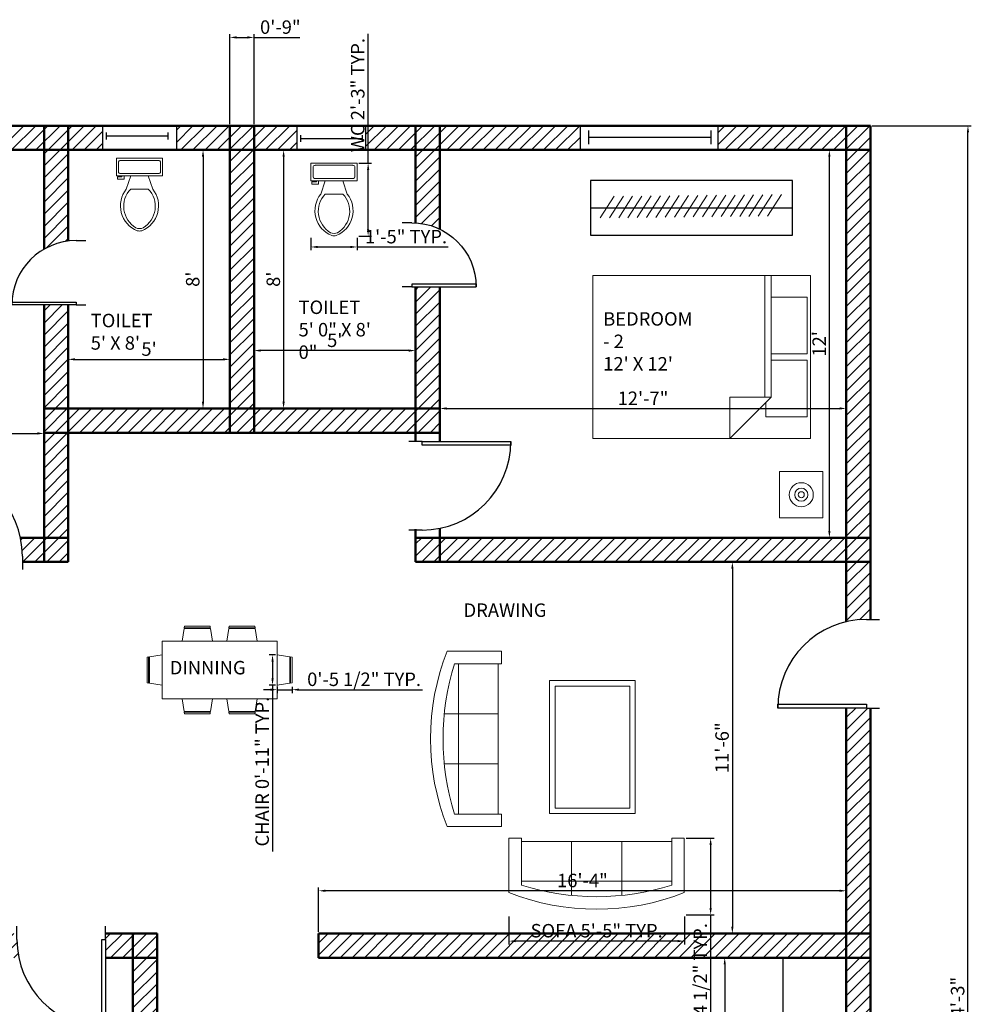
# Model space of a CAD drawing. Units: millimetres. Extents: x 2829 to 4029, y 962 to 1687.
# Tile 7 of 7: x 3676 to 4029, y 1321 to 1687. Entities that reach past the tile are written whole.
import ezdxf

# ---------------------------------------------------------------- set-up
doc = ezdxf.new("R2010")
doc.units = ezdxf.units.MM
for name, color, linetype, lineweight in [('A-ANNO-DIMS', 140, 'Continuous', 18), ('A-AREA-IDEN', 190, 'Continuous', 25), ('A-FLOR-CASE', 90, 'Continuous', 25), ('A-FLOR-CASE-PATT', 90, 'Continuous', 13), ('A-FLOR-FIXT', 90, 'Continuous', 18), ('A-WALL-PATT', 2, 'Continuous', 13), ('doors', 10, 'Continuous', 25), ('furniture', 90, 'Continuous', 18), ('walls', 50, 'Continuous', 50), ('windows', 30, 'Continuous', 25)]:
    doc.layers.add(name, color=color, linetype=linetype, lineweight=lineweight)
doc.styles.get("Standard").update_dxf_attribs({"font": 'arial.ttf'})
doc.dimstyles.new('ISO-25', dxfattribs={"dimtxt": 5, "dimasz": 2.5, "dimexe": 1.25, "dimexo": 0.625, "dimtad": 1, "dimdec": 0, "dimlunit": 3, "dimtxsty": 'Standard', "dimcen": 2.5, "dimadec": 0, "dimazin": 0, "dimtfac": 1, "dimtdec": 0, "dimtmove": 0, "dimatfit": 3, "dimfxl": 1, "dimarcsym": 0})
pattern_1 = [(45, (-1090.0668, 570.9627), (-2.245064, 2.245064), [])]

# ---------------------------------------------------------------- blocks, each defined once
blk = doc.blocks.new('*U2')
for p, q in [((0, 0), (0, -6)), ((40, 0), (40, -6))]:
    blk.add_line(p, q)
blk.add_lwpolyline([(0, 0), (0, 40), (1.75, 40), (1.75, 0)], close=True)
blk.add_arc((0, 0), 40, 0, 90)
blk = doc.blocks.new('*U32')
for p, q in [((0, 4), (0, 0)), ((36, 4), (36, 0)), ((0, 2), (36, 2))]:
    blk.add_line(p, q)
blk = doc.blocks.new('*U33')
for p, q in [((0, 4), (0, 0)), ((0, 2), (36, 2)), ((36, 4), (36, 0))]:
    blk.add_line(p, q)
blk = doc.blocks.new('Bed - Queen')
for p, q in [((0, -80.00003), (0, 0)), ((0, 0), (59.99999, 0)), ((59.99999, 0), (59.99999, -80.00003)), ((7.99999, -1.2), (28.79998, -1.2)), ((7.99999, -14.4), (7.99999, -1.2)), ((28.79998, -1.2), (28.79998, -14.4)), ((31.19999, -1.2), (51.99999, -1.2)), ((31.19999, -14.4), (31.19999, -1.2)), ((51.99999, -1.2), (51.99999, -16.4)), ((0, -14.4), (44.8, -14.4)), ((59.99999, -29.6), (44.8, -14.4)), ((44.8, -14.4), (44.8, -29.6)), ((44.8, -16.8), (0, -16.8)), ((51.99999, -16.4), (46.79936, -16.4)), ((44.8, -29.6), (59.99999, -29.6)), ((59.99999, -80.00003), (0, -80.00003))]:
    blk.add_line(p, q)
blk = doc.blocks.new('Sofa - Roundback 7 ft.')
for p, q in [((-12.00002, -32.4421), (-12.00003, -6.5971)), ((11.99997, -32.4421), (11.99998, -6.5971)), ((-36.000027, -34), (-36.000027, -11.4696)), ((-35.999844, -13.3819), (35.9998, -13.3819)), ((35.99998, -34), (35.99998, -11.4696)), ((-36.000027, -32.4421), (35.99998, -32.4421))]:
    blk.add_line(p, q)
for points in [[(-36.000027, -34), (-42.000027, -34), (-42.000027, -8)], [(41.99998, -8), (41.99998, -34), (35.99998, -34)]]:
    blk.add_lwpolyline(points)
for centre, radius, start, end in [((0, -114.25), 114.25, 68.43141, 111.5686), ((-0.00001, -127.1968), 121.1968, 72.72033, 107.2797)]:
    blk.add_arc(centre, radius, start, end)
blk = doc.blocks.new('Toilet - top')
for p, q in [((9.5, -6), (9.5, -2)), ((-10, -8.5), (-8, -8.5)), ((-10, -9.5), (-10, -8.5)), ((-8, -8.5), (-8, -8)), ((-7, -8), (-7, -9.5)), ((-4, -8), (-6, -14)), ((4, -8), (6, -14)), ((-7, -9.5), (-10, -9.5)), ((4, -14), (-4, -14))]:
    blk.add_line(p, q)
blk.add_lwpolyline([(10.5, -8), (10.5, 0), (-10.5, 0), (-10.5, -8)], close=True)
for points in [[(-9.5, -2), (-9.5, -6)], [(8.5, -1), (-8.5, -1)], [(-8.5, -7), (8.5, -7)]]:
    blk.add_lwpolyline(points)
for centre, radius, start, end in [((-8.62, -1.88), 0.884, 81.8699, 188.1301), ((8.62, -1.88), 0.884, 351.8699, 98.1301), ((-8.62, -6.12), 0.884, 171.8699, 278.1301), ((8.62, -6.12), 0.884, 261.8699, 8.1301), ((3.52, -21.58), 12.17, 141.4691, 247.9714), ((4.2, -21.82), 11.33, 136.3677, 238.9468), ((-3.52, -21.58), 12.17, 292.0284, 38.5307), ((-4.2, -21.82), 11.33, 301.053, 43.6321), ((0, -27.88), 4, 245.7318, 294.2682), ((0, -29), 4, 254.8605, 285.1395)]:
    blk.add_arc(centre, radius, start, end)
blk = doc.blocks.new('*D36')
at = {"layer": 'A-ANNO-DIMS', "color": 0, "lineweight": -2, "transparency": 16777216}
for p, q in [((3533.66, 1539.68), (3533.66, 1531.75)), ((3684.66, 1539.68), (3684.66, 1531.75)), ((3536.16, 1533), (3682.16, 1533))]:
    blk.add_line(p, q, dxfattribs=at)
at = {"layer": 'A-ANNO-DIMS', "color": 0, "transparency": 16777216}
for points in [[(3536.16, 1533.42), (3536.16, 1532.59), (3533.66, 1533)], [(3682.16, 1533.42), (3682.16, 1532.59), (3684.66, 1533)]]:
    blk.add_solid(points, dxfattribs=at)
at = {"layer": 'Defpoints', "color": 0, "transparency": 16777216}
for p in [(3533.66, 1540.3), (3684.66, 1540.3), (3684.66, 1533)]:
    blk.add_point(p, dxfattribs=at)
at = {"layer": 'A-ANNO-DIMS', "color": 0, "transparency": 16777216, "insert": (3609.16, 1536.14), "char_height": 5, "attachment_point": 5}
blk.add_mtext('12\'-7"', dxfattribs=at)
blk = doc.blocks.new('*D38')
at = {"layer": 'A-ANNO-DIMS', "color": 0, "lineweight": -2, "transparency": 16777216}
for p, q in [((3744.35, 1638.27), (3744.97, 1638.27)), ((3743.72, 1635.77), (3743.72, 1544.77)), ((3744.35, 1542.27), (3744.97, 1542.27))]:
    blk.add_line(p, q, dxfattribs=at)
at = {"layer": 'A-ANNO-DIMS', "color": 0, "transparency": 16777216}
for points in [[(3743.3, 1635.77), (3744.14, 1635.77), (3743.72, 1638.27)], [(3743.3, 1544.77), (3744.14, 1544.77), (3743.72, 1542.27)]]:
    blk.add_solid(points, dxfattribs=at)
at = {"layer": 'Defpoints', "color": 0, "transparency": 16777216}
for p in [(3743.72, 1638.27), (3743.72, 1542.27), (3743.72, 1542.27)]:
    blk.add_point(p, dxfattribs=at)
at = {"layer": 'A-ANNO-DIMS', "color": 0, "transparency": 16777216, "insert": (3740.54, 1590.27), "char_height": 5, "attachment_point": 5, "rotation": 90}
blk.add_mtext("8'", dxfattribs=at)
blk = doc.blocks.new('*D39')
at = {"layer": 'A-ANNO-DIMS', "color": 0, "lineweight": -2, "transparency": 16777216}
for p, q in [((3693.66, 1556.42), (3693.66, 1561.76)), ((3753.66, 1556.42), (3753.66, 1561.76)), ((3696.16, 1560.51), (3751.16, 1560.51))]:
    blk.add_line(p, q, dxfattribs=at)
at = {"layer": 'A-ANNO-DIMS', "color": 0, "transparency": 16777216}
for points in [[(3696.16, 1560.92), (3696.16, 1560.09), (3693.66, 1560.51)], [(3751.16, 1560.92), (3751.16, 1560.09), (3753.66, 1560.51)]]:
    blk.add_solid(points, dxfattribs=at)
at = {"layer": 'Defpoints', "color": 0, "transparency": 16777216}
for p in [(3753.66, 1560.51), (3693.66, 1555.8), (3753.66, 1555.8)]:
    blk.add_point(p, dxfattribs=at)
at = {"layer": 'A-ANNO-DIMS', "color": 0, "transparency": 16777216, "insert": (3723.66, 1563.67), "char_height": 5, "attachment_point": 5}
blk.add_mtext("5'", dxfattribs=at)
blk = doc.blocks.new('*D40')
at = {"layer": 'A-ANNO-DIMS', "color": 0, "lineweight": -2, "transparency": 16777216}
for p, q in [((3774.27, 1638.27), (3774.9, 1638.27)), ((3773.65, 1635.77), (3773.65, 1544.77)), ((3774.27, 1542.27), (3774.9, 1542.27))]:
    blk.add_line(p, q, dxfattribs=at)
at = {"layer": 'A-ANNO-DIMS', "color": 0, "transparency": 16777216}
for points in [[(3773.23, 1635.77), (3774.07, 1635.77), (3773.65, 1638.27)], [(3773.23, 1544.77), (3774.07, 1544.77), (3773.65, 1542.27)]]:
    blk.add_solid(points, dxfattribs=at)
at = {"layer": 'Defpoints', "color": 0, "transparency": 16777216}
for p in [(3773.65, 1638.27), (3773.65, 1542.27), (3773.65, 1542.27)]:
    blk.add_point(p, dxfattribs=at)
at = {"layer": 'A-ANNO-DIMS', "color": 0, "transparency": 16777216, "insert": (3770.47, 1590.27), "char_height": 5, "attachment_point": 5, "rotation": 90}
blk.add_mtext("8'", dxfattribs=at)
blk = doc.blocks.new('*D41')
at = {"layer": 'A-ANNO-DIMS', "color": 0, "lineweight": -2, "transparency": 16777216}
for p, q in [((3762.66, 1564.4), (3762.66, 1565.02)), ((3820.16, 1563.77), (3765.16, 1563.77)), ((3822.66, 1564.4), (3822.66, 1565.02))]:
    blk.add_line(p, q, dxfattribs=at)
at = {"layer": 'A-ANNO-DIMS', "color": 0, "transparency": 16777216}
for points in [[(3765.16, 1564.19), (3765.16, 1563.35), (3762.66, 1563.77)], [(3820.16, 1564.19), (3820.16, 1563.35), (3822.66, 1563.77)]]:
    blk.add_solid(points, dxfattribs=at)
at = {"layer": 'Defpoints', "color": 0, "transparency": 16777216}
for p in [(3762.66, 1563.77), (3762.66, 1563.77), (3822.66, 1563.77)]:
    blk.add_point(p, dxfattribs=at)
at = {"layer": 'A-ANNO-DIMS', "color": 0, "transparency": 16777216, "insert": (3792.66, 1566.94), "char_height": 5, "attachment_point": 5}
blk.add_mtext("5'", dxfattribs=at)
blk = doc.blocks.new('*D53')
at = {"layer": 'A-ANNO-DIMS', "color": 0, "lineweight": -2, "transparency": 16777216}
for p, q in [((3940.98, 1485.27), (3941.6, 1485.27)), ((3940.35, 1482.77), (3940.35, 1349.77)), ((3940.98, 1347.27), (3941.6, 1347.27))]:
    blk.add_line(p, q, dxfattribs=at)
at = {"layer": 'A-ANNO-DIMS', "color": 0, "transparency": 16777216}
for points in [[(3939.94, 1482.77), (3940.77, 1482.77), (3940.35, 1485.27)], [(3939.94, 1349.77), (3940.77, 1349.77), (3940.35, 1347.27)]]:
    blk.add_solid(points, dxfattribs=at)
at = {"layer": 'Defpoints', "color": 0, "transparency": 16777216}
for p in [(3940.35, 1485.27), (3940.35, 1347.27), (3940.35, 1347.27)]:
    blk.add_point(p, dxfattribs=at)
at = {"layer": 'A-ANNO-DIMS', "color": 0, "transparency": 16777216, "insert": (3937.17, 1416.27), "char_height": 5, "attachment_point": 5, "rotation": 90}
blk.add_mtext('11\'-6"', dxfattribs=at)
blk = doc.blocks.new('*D54')
at = {"layer": 'A-ANNO-DIMS', "color": 0, "lineweight": -2, "transparency": 16777216}
for p, q in [((3786.66, 1347.9), (3786.66, 1364.4)), ((3982.66, 1354.73), (3982.66, 1364.4)), ((3980.16, 1363.15), (3789.16, 1363.15))]:
    blk.add_line(p, q, dxfattribs=at)
at = {"layer": 'A-ANNO-DIMS', "color": 0, "transparency": 16777216}
for points in [[(3789.16, 1363.56), (3789.16, 1362.73), (3786.66, 1363.15)], [(3980.16, 1363.56), (3980.16, 1362.73), (3982.66, 1363.15)]]:
    blk.add_solid(points, dxfattribs=at)
at = {"layer": 'Defpoints', "color": 0, "transparency": 16777216}
for p in [(3786.66, 1363.15), (3982.66, 1354.11), (3786.66, 1347.27)]:
    blk.add_point(p, dxfattribs=at)
at = {"layer": 'A-ANNO-DIMS', "color": 0, "transparency": 16777216, "insert": (3884.66, 1366.32), "char_height": 5, "attachment_point": 5}
blk.add_mtext('16\'-4"', dxfattribs=at)
blk = doc.blocks.new('*D55')
at = {"layer": 'A-ANNO-DIMS', "color": 0, "lineweight": -2, "transparency": 16777216}
for p, q in [((3937.54, 1338.27), (3936.26, 1338.27)), ((3937.51, 1335.77), (3937.51, 1196.77)), ((3937.54, 1194.27), (3936.26, 1194.27))]:
    blk.add_line(p, q, dxfattribs=at)
at = {"layer": 'A-ANNO-DIMS', "color": 0, "transparency": 16777216}
for points in [[(3937.1, 1335.77), (3937.93, 1335.77), (3937.51, 1338.27)], [(3937.1, 1196.77), (3937.93, 1196.77), (3937.51, 1194.27)]]:
    blk.add_solid(points, dxfattribs=at)
at = {"layer": 'Defpoints', "color": 0, "transparency": 16777216}
for p in [(3938.16, 1338.27), (3937.51, 1194.27), (3938.16, 1194.27)]:
    blk.add_point(p, dxfattribs=at)
at = {"layer": 'A-ANNO-DIMS', "color": 0, "transparency": 16777216, "insert": (3934.38, 1266.27), "char_height": 5, "attachment_point": 5, "rotation": 90}
blk.add_mtext("12'", dxfattribs=at)
blk = doc.blocks.new('*D57')
at = {"layer": 'A-ANNO-DIMS', "color": 0, "lineweight": -2, "transparency": 16777216}
for p, q in [((3977.01, 1638.27), (3977.64, 1638.27)), ((3976.39, 1496.77), (3976.39, 1635.77)), ((3977.01, 1494.27), (3977.64, 1494.27))]:
    blk.add_line(p, q, dxfattribs=at)
at = {"layer": 'A-ANNO-DIMS', "color": 0, "transparency": 16777216}
for points in [[(3975.97, 1635.77), (3976.81, 1635.77), (3976.39, 1638.27)], [(3975.97, 1496.77), (3976.81, 1496.77), (3976.39, 1494.27)]]:
    blk.add_solid(points, dxfattribs=at)
at = {"layer": 'Defpoints', "color": 0, "transparency": 16777216}
for p in [(3976.39, 1638.27), (3976.39, 1638.27), (3976.39, 1494.27)]:
    blk.add_point(p, dxfattribs=at)
at = {"layer": 'A-ANNO-DIMS', "color": 0, "transparency": 16777216, "insert": (3973.25, 1566.27), "char_height": 5, "attachment_point": 5, "rotation": 90}
blk.add_mtext("12'", dxfattribs=at)
blk = doc.blocks.new('*D58')
at = {"layer": 'A-ANNO-DIMS', "color": 0, "lineweight": -2, "transparency": 16777216}
for p, q in [((3831.66, 1542.9), (3831.66, 1543.52)), ((3982.66, 1542.9), (3982.66, 1543.52)), ((3834.16, 1542.27), (3980.16, 1542.27))]:
    blk.add_line(p, q, dxfattribs=at)
at = {"layer": 'A-ANNO-DIMS', "color": 0, "transparency": 16777216}
for points in [[(3834.16, 1542.69), (3834.16, 1541.85), (3831.66, 1542.27)], [(3980.16, 1542.69), (3980.16, 1541.85), (3982.66, 1542.27)]]:
    blk.add_solid(points, dxfattribs=at)
at = {"layer": 'Defpoints', "color": 0, "transparency": 16777216}
for p in [(3831.66, 1542.27), (3982.66, 1542.27), (3982.66, 1542.27)]:
    blk.add_point(p, dxfattribs=at)
at = {"layer": 'A-ANNO-DIMS', "color": 0, "transparency": 16777216, "insert": (3907.16, 1545.41), "char_height": 5, "attachment_point": 5}
blk.add_mtext('12\'-7"', dxfattribs=at)
blk = doc.blocks.new('CHAIR-DINING')
for p, q in [((0.74, 4.74), (0, 0)), ((0.74, 4.74), (10.5, 4.74)), ((0.88, 5.63), (0.79, 5.04)), ((10.46, 5.04), (0.79, 5.04)), ((0.88, 5.63), (10.36, 5.63)), ((10.46, 5.04), (10.36, 5.63)), ((11.24, 0), (10.5, 4.74))]:
    blk.add_line(p, q)
blk = doc.blocks.new('*D67')
at = {"layer": 'A-ANNO-DIMS', "color": 0, "lineweight": -2, "transparency": 16777216}
for p, q in [((3857.36, 1353.61), (3857.36, 1343.21)), ((3922.51, 1353.61), (3922.51, 1343.21)), ((3920.01, 1344.46), (3859.86, 1344.46))]:
    blk.add_line(p, q, dxfattribs=at)
at = {"layer": 'A-ANNO-DIMS', "color": 0, "transparency": 16777216}
for points in [[(3859.86, 1344.88), (3859.86, 1344.04), (3857.36, 1344.46)], [(3920.01, 1344.88), (3920.01, 1344.04), (3922.51, 1344.46)]]:
    blk.add_solid(points, dxfattribs=at)
at = {"layer": 'Defpoints', "color": 0, "transparency": 16777216}
for p in [(3857.36, 1354.23), (3922.51, 1354.23), (3857.36, 1344.46)]:
    blk.add_point(p, dxfattribs=at)
at = {"layer": 'A-ANNO-DIMS', "color": 0, "transparency": 16777216, "insert": (3889.93, 1347.67), "char_height": 5, "attachment_point": 5}
blk.add_mtext('SOFA 5\'-5" TYP.', dxfattribs=at)
blk = doc.blocks.new('*D68')
at = {"layer": 'A-ANNO-DIMS', "color": 0, "lineweight": -2, "transparency": 16777216}
for p, q in [((3923.13, 1382.67), (3933.53, 1382.67)), ((3932.28, 1380.17), (3932.28, 1356.73)), ((3923.13, 1354.23), (3933.53, 1354.23)), ((3932.28, 1354.23), (3932.28, 1308.27))]:
    blk.add_line(p, q, dxfattribs=at)
at = {"layer": 'A-ANNO-DIMS', "color": 0, "transparency": 16777216}
for points in [[(3931.86, 1380.17), (3932.7, 1380.17), (3932.28, 1382.67)], [(3931.86, 1356.73), (3932.7, 1356.73), (3932.28, 1354.23)]]:
    blk.add_solid(points, dxfattribs=at)
at = {"layer": 'Defpoints', "color": 0, "transparency": 16777216}
for p in [(3922.51, 1382.67), (3922.51, 1354.23), (3932.28, 1354.23)]:
    blk.add_point(p, dxfattribs=at)
at = {"layer": 'A-ANNO-DIMS', "color": 0, "transparency": 16777216, "insert": (3929.07, 1330), "char_height": 5, "attachment_point": 5, "rotation": 90}
blk.add_mtext('2\'-4 1/2" TYP.', dxfattribs=at)
blk = doc.blocks.new('*D75')
at = {"layer": 'A-ANNO-DIMS', "color": 0, "lineweight": -2, "transparency": 16777216}
for p, q in [((3805.04, 1633.39), (3805.04, 1681.4)), ((3801.61, 1633.39), (3806.29, 1633.39)), ((3805.04, 1608.81), (3805.04, 1630.89)), ((3801.61, 1606.31), (3806.29, 1606.31))]:
    blk.add_line(p, q, dxfattribs=at)
at = {"layer": 'A-ANNO-DIMS', "color": 0, "transparency": 16777216}
for points in [[(3804.63, 1630.89), (3805.46, 1630.89), (3805.04, 1633.39)], [(3804.63, 1608.81), (3805.46, 1608.81), (3805.04, 1606.31)]]:
    blk.add_solid(points, dxfattribs=at)
at = {"layer": 'Defpoints', "color": 0, "transparency": 16777216}
for p in [(3800.98, 1633.39), (3805.04, 1633.39), (3800.98, 1606.31)]:
    blk.add_point(p, dxfattribs=at)
at = {"layer": 'A-ANNO-DIMS', "color": 0, "transparency": 16777216, "insert": (3801.83, 1658.65), "char_height": 5, "attachment_point": 5, "rotation": 90}
blk.add_mtext('WC 2\'-3" TYP.', dxfattribs=at)
blk = doc.blocks.new('*D76')
at = {"layer": 'A-ANNO-DIMS', "color": 0, "lineweight": -2, "transparency": 16777216}
for p, q in [((3783.78, 1605.69), (3783.78, 1601)), ((3800.98, 1605.69), (3800.98, 1601)), ((3786.28, 1602.25), (3798.48, 1602.25)), ((3800.98, 1602.25), (3834.74, 1602.25))]:
    blk.add_line(p, q, dxfattribs=at)
at = {"layer": 'A-ANNO-DIMS', "color": 0, "transparency": 16777216}
for points in [[(3786.28, 1602.67), (3786.28, 1601.84), (3783.78, 1602.25)], [(3798.48, 1602.67), (3798.48, 1601.84), (3800.98, 1602.25)]]:
    blk.add_solid(points, dxfattribs=at)
at = {"layer": 'Defpoints', "color": 0, "transparency": 16777216}
for p in [(3783.78, 1606.31), (3800.98, 1606.31), (3800.98, 1602.25)]:
    blk.add_point(p, dxfattribs=at)
at = {"layer": 'A-ANNO-DIMS', "color": 0, "transparency": 16777216, "insert": (3819.11, 1605.43), "char_height": 5, "attachment_point": 5}
blk.add_mtext('1\'-5" TYP.', dxfattribs=at)
blk = doc.blocks.new('*D77')
at = {"layer": 'A-ANNO-DIMS', "color": 0, "lineweight": -2, "transparency": 16777216}
for p, q in [((3770.6, 1450.76), (3768.29, 1450.76)), ((3769.54, 1448.26), (3769.54, 1442.01)), ((3770.6, 1439.51), (3768.29, 1439.51)), ((3769.54, 1439.51), (3769.54, 1377.78))]:
    blk.add_line(p, q, dxfattribs=at)
at = {"layer": 'A-ANNO-DIMS', "color": 0, "transparency": 16777216}
for points in [[(3769.13, 1448.26), (3769.96, 1448.26), (3769.54, 1450.76)], [(3769.13, 1442.01), (3769.96, 1442.01), (3769.54, 1439.51)]]:
    blk.add_solid(points, dxfattribs=at)
at = {"layer": 'Defpoints', "color": 0, "transparency": 16777216}
for p in [(3771.23, 1450.76), (3769.54, 1439.51), (3771.23, 1439.51)]:
    blk.add_point(p, dxfattribs=at)
at = {"layer": 'A-ANNO-DIMS', "color": 0, "transparency": 16777216, "insert": (3766.33, 1407.4), "char_height": 5, "attachment_point": 5, "rotation": 90}
blk.add_mtext('CHAIR 0\'-11" TYP.', dxfattribs=at)
blk = doc.blocks.new('*D78')
at = {"layer": 'A-ANNO-DIMS', "color": 0, "lineweight": -2, "transparency": 16777216}
for p, q in [((3768.73, 1437.83), (3766.23, 1437.83)), ((3771.23, 1438.89), (3771.23, 1436.58)), ((3771.23, 1437.83), (3776.86, 1437.83)), ((3776.86, 1438.89), (3776.86, 1436.58)), ((3779.36, 1437.83), (3825.24, 1437.83))]:
    blk.add_line(p, q, dxfattribs=at)
at = {"layer": 'A-ANNO-DIMS', "color": 0, "transparency": 16777216}
for points in [[(3768.73, 1438.24), (3768.73, 1437.41), (3771.23, 1437.83)], [(3779.36, 1438.24), (3779.36, 1437.41), (3776.86, 1437.83)]]:
    blk.add_solid(points, dxfattribs=at)
at = {"layer": 'Defpoints', "color": 0, "transparency": 16777216}
for p in [(3771.23, 1439.51), (3776.86, 1439.51), (3776.86, 1437.83)]:
    blk.add_point(p, dxfattribs=at)
at = {"layer": 'A-ANNO-DIMS', "color": 0, "transparency": 16777216, "insert": (3803.55, 1441.04), "char_height": 5, "attachment_point": 5}
blk.add_mtext('0\'-5 1/2" TYP.', dxfattribs=at)
blk = doc.blocks.new('*D92')
at = {"layer": 'A-ANNO-DIMS', "color": 0, "lineweight": -2, "transparency": 16777216}
for p, q in [((3443.66, 1337.65), (3443.66, 962.22)), ((3991.66, 995.65), (3991.66, 962.22)), ((3446.16, 963.47), (3989.16, 963.47))]:
    blk.add_line(p, q, dxfattribs=at)
at = {"layer": 'A-ANNO-DIMS', "color": 0, "transparency": 16777216}
for points in [[(3446.16, 963.89), (3446.16, 963.05), (3443.66, 963.47)], [(3989.16, 963.89), (3989.16, 963.05), (3991.66, 963.47)]]:
    blk.add_solid(points, dxfattribs=at)
at = {"layer": 'Defpoints', "color": 0, "transparency": 16777216}
for p in [(3443.66, 1338.27), (3991.66, 996.27), (3991.66, 963.47)]:
    blk.add_point(p, dxfattribs=at)
at = {"layer": 'A-ANNO-DIMS', "color": 0, "transparency": 16777216, "insert": (3717.66, 966.65), "char_height": 5, "attachment_point": 5}
blk.add_mtext('45\'-8"', dxfattribs=at)
blk = doc.blocks.new('*D93')
at = {"layer": 'A-ANNO-DIMS', "color": 0, "lineweight": -2, "transparency": 16777216}
for p, q in [((3992.28, 1647.27), (4029.11, 1647.27)), ((4027.86, 998.77), (4027.86, 1644.77)), ((3992.28, 996.27), (4029.11, 996.27))]:
    blk.add_line(p, q, dxfattribs=at)
at = {"layer": 'A-ANNO-DIMS', "color": 0, "transparency": 16777216}
for points in [[(4027.44, 1644.77), (4028.28, 1644.77), (4027.86, 1647.27)], [(4027.44, 998.77), (4028.28, 998.77), (4027.86, 996.27)]]:
    blk.add_solid(points, dxfattribs=at)
at = {"layer": 'Defpoints', "color": 0, "transparency": 16777216}
for p in [(3991.66, 1647.27), (4027.86, 1647.27), (3991.66, 996.27)]:
    blk.add_point(p, dxfattribs=at)
at = {"layer": 'A-ANNO-DIMS', "color": 0, "transparency": 16777216, "insert": (4024.68, 1321.77), "char_height": 5, "attachment_point": 5, "rotation": 90}
blk.add_mtext('54\'-3"', dxfattribs=at)
blk = doc.blocks.new('*D95')
at = {"layer": 'A-ANNO-DIMS', "color": 0, "lineweight": -2, "transparency": 16777216}
for p, q in [((3753.66, 1647.9), (3753.66, 1681.32)), ((3756.16, 1680.07), (3760.16, 1680.07)), ((3762.66, 1647.9), (3762.66, 1681.32)), ((3762.66, 1680.07), (3779.7, 1680.07))]:
    blk.add_line(p, q, dxfattribs=at)
at = {"layer": 'A-ANNO-DIMS', "color": 0, "transparency": 16777216}
for points in [[(3756.16, 1680.49), (3756.16, 1679.65), (3753.66, 1680.07)], [(3760.16, 1680.49), (3760.16, 1679.65), (3762.66, 1680.07)]]:
    blk.add_solid(points, dxfattribs=at)
at = {"layer": 'Defpoints', "color": 0, "transparency": 16777216}
for p in [(3762.66, 1680.07), (3753.66, 1647.27), (3762.66, 1647.27)]:
    blk.add_point(p, dxfattribs=at)
at = {"layer": 'A-ANNO-DIMS', "color": 0, "transparency": 16777216, "insert": (3772.43, 1683.25), "char_height": 5, "attachment_point": 5}
blk.add_mtext('0\'-9"', dxfattribs=at)

msp = doc.modelspace()

# ---------------------------------------------------------------- hatches: boundary and pattern name
at = {"layer": 'A-FLOR-CASE-PATT'}
h = msp.add_hatch(dxfattribs=at)
h.set_pattern_fill('ANSI31', color=256, scale=0.908318, angle=12.144, style=0)
h.paths.add_polyline_path([(3889.26, 1612.99), (3954.95, 1613.71), (3960.15, 1621.75), (3894.46, 1621.04)])
at = {"layer": 'A-WALL-PATT'}
h = msp.add_hatch(dxfattribs=at)
h.set_pattern_fill('ANSI31', color=256)
h.set_pattern_definition(pattern_1)
h.paths.add_polyline_path([(3524.66, 1494.27), (3452.66, 1494.27), (3452.66, 1485.27), (3524.66, 1485.27)])
h.paths.add_polyline_path([(3452.66, 1494.27), (3443.66, 1494.27), (3443.66, 1485.27), (3452.66, 1485.27)])
h.paths.add_polyline_path([(3452.66, 1485.27), (3443.66, 1485.27), (3443.66, 1347.27), (3452.66, 1347.27)])
h.paths.add_polyline_path([(3533.66, 1433.28), (3524.66, 1433.28), (3524.66, 1400.41), (3533.66, 1400.41)])
h.paths.add_polyline_path([(3524.66, 1347.27), (3452.66, 1347.27), (3452.66, 1338.27), (3524.66, 1338.27)])
h.paths.add_polyline_path([(3452.66, 1347.27), (3443.66, 1347.27), (3443.66, 1338.27), (3452.66, 1338.27)])
h.paths.add_polyline_path([(3533.66, 1347.27), (3524.66, 1347.27), (3524.66, 1338.27), (3533.66, 1338.27)])
h.paths.add_polyline_path([(3674.61, 1345.02), (3674.61, 1347.27), (3533.66, 1347.27), (3533.66, 1338.27), (3675.31, 1338.27, -0.051672)])
h.paths.add_polyline_path([(3533.66, 1638.27), (3524.66, 1638.27), (3524.66, 1494.27), (3533.66, 1494.27)])
h.paths.add_polyline_path([(3533.66, 1494.27), (3524.66, 1494.27), (3524.66, 1485.27), (3533.66, 1485.27)])
h.paths.add_polyline_path([(3643.72, 1494.27), (3533.66, 1494.27), (3533.66, 1485.27), (3643.72, 1485.27), (3643.72, 1487.41)])
h.paths.add_polyline_path([(3533.66, 1647.27), (3524.66, 1647.27), (3524.66, 1638.27), (3533.66, 1638.27)])
h.paths.add_polyline_path([(3573.07, 1647.27), (3533.66, 1647.27), (3533.66, 1638.27), (3573.07, 1638.27)])
h.paths.add_polyline_path([(3684.66, 1647.27), (3622.32, 1647.27), (3622.32, 1638.27), (3684.66, 1638.27)])
h.paths.add_polyline_path([(3693.66, 1647.27), (3684.66, 1647.27), (3684.66, 1638.27), (3693.66, 1638.27)])
h.paths.add_polyline_path([(3693.66, 1638.27), (3684.66, 1638.27), (3684.66, 1601.42, -0.100401), (3693.66, 1604.42)])
h.paths.add_polyline_path([(3693.66, 1580.73), (3684.66, 1580.73), (3684.66, 1542.27), (3693.66, 1542.27)])
h.paths.add_polyline_path([(3693.66, 1542.27), (3684.66, 1542.27), (3684.66, 1533.27), (3693.66, 1533.27)])
h.paths.add_polyline_path([(3693.66, 1533.27), (3684.66, 1533.27), (3684.66, 1494.27), (3693.66, 1494.27)])
h.paths.add_polyline_path([(3693.66, 1494.27), (3684.66, 1494.27), (3684.66, 1485.27), (3693.66, 1485.27)])
h.paths.add_polyline_path([(3684.66, 1494.27), (3675.91, 1494.27, -0.052559), (3676.64, 1487.41), (3676.64, 1485.27), (3684.66, 1485.27)])
h.paths.add_polyline_path([(3753.66, 1542.27), (3693.66, 1542.27), (3693.66, 1533.27), (3753.66, 1533.27)])
h.paths.add_polyline_path([(3762.66, 1542.27), (3753.66, 1542.27), (3753.66, 1533.27), (3762.66, 1533.27)])
h.paths.add_polyline_path([(3762.66, 1638.27), (3753.66, 1638.27), (3753.66, 1542.27), (3762.66, 1542.27)])
h.paths.add_polyline_path([(3762.66, 1647.27), (3753.66, 1647.27), (3753.66, 1638.27), (3762.66, 1638.27)])
h.paths.add_polyline_path([(3753.66, 1647.27), (3733.82, 1647.27), (3733.82, 1638.27), (3753.66, 1638.27)])
h.paths.add_polyline_path([(3706.41, 1647.27), (3693.66, 1647.27), (3693.66, 1638.27), (3706.41, 1638.27)])
h.paths.add_polyline_path([(3822.66, 1647.27), (3804.07, 1647.27), (3804.07, 1638.27), (3822.66, 1638.27)])
h.paths.add_polyline_path([(3778.61, 1647.27), (3762.66, 1647.27), (3762.66, 1638.27), (3778.61, 1638.27)])
h.paths.add_polyline_path([(3822.66, 1542.27), (3762.66, 1542.27), (3762.66, 1533.27), (3822.66, 1533.27)])
h.paths.add_polyline_path([(3831.66, 1542.27), (3822.66, 1542.27), (3822.66, 1533.27), (3831.66, 1533.27)])
h.paths.add_polyline_path([(3831.66, 1587.4), (3822.66, 1587.4), (3822.66, 1542.27), (3831.66, 1542.27)])
h.paths.add_polyline_path([(3831.66, 1638.27), (3822.66, 1638.27), (3822.66, 1611.22, -0.098322), (3831.66, 1608.9)])
h.paths.add_polyline_path([(3831.66, 1647.27), (3822.66, 1647.27), (3822.66, 1638.27), (3831.66, 1638.27)])
h.paths.add_polyline_path([(3883.77, 1647.27), (3831.66, 1647.27), (3831.66, 1638.27), (3883.77, 1638.27)])
h.paths.add_polyline_path([(3982.66, 1647.27), (3934.96, 1647.27), (3934.96, 1638.27), (3982.66, 1638.27)])
h.paths.add_polyline_path([(3991.66, 1647.27), (3982.66, 1647.27), (3982.66, 1638.27), (3991.66, 1638.27)])
h.paths.add_polyline_path([(3991.66, 1638.27), (3982.66, 1638.27), (3982.66, 1494.27), (3991.66, 1494.27)])
h.paths.add_polyline_path([(3991.66, 1494.27), (3982.66, 1494.27), (3982.66, 1485.27), (3991.66, 1485.27)])
h.paths.add_polyline_path([(3982.66, 1494.27), (3831.66, 1494.27), (3831.66, 1485.27), (3982.66, 1485.27)])
h.paths.add_polyline_path([(3831.66, 1494.27), (3822.66, 1494.27), (3822.66, 1485.27), (3831.66, 1485.27)])
h.paths.add_polyline_path([(3991.66, 1485.27), (3982.66, 1485.27), (3982.66, 1463.05, -0.057246), (3990.12, 1463.9), (3991.66, 1463.9)])
h.paths.add_polyline_path([(3991.66, 1430.98), (3990.12, 1430.98), (3982.66, 1430.98), (3982.66, 1347.27), (3991.66, 1347.27)])
h.paths.add_polyline_path([(3982.66, 1347.27), (3786.66, 1347.27), (3786.66, 1338.27), (3982.66, 1338.27)])
h.paths.add_polyline_path([(3991.66, 1347.27), (3982.66, 1347.27), (3982.66, 1338.27), (3991.66, 1338.27)])
h.paths.add_polyline_path([(3991.66, 1338.27), (3982.66, 1338.27), (3982.66, 1005.27), (3991.66, 1005.27)])
h.paths.add_polyline_path([(3982.66, 1194.27), (3879.62, 1194.27), (3879.62, 1185.27), (3982.66, 1185.27)])
h.paths.add_polyline_path([(3853.79, 1194.27), (3795.66, 1194.27), (3795.66, 1185.27), (3853.79, 1185.27)])
h.paths.add_polyline_path([(3795.66, 1194.27), (3786.66, 1194.27), (3786.66, 1185.27), (3795.66, 1185.27)])
h.paths.add_polyline_path([(3795.66, 1290.27), (3786.66, 1290.27), (3786.66, 1194.27), (3795.66, 1194.27)])
h.paths.add_polyline_path([(3726.66, 1230.69), (3717.66, 1230.69), (3717.66, 1194.27), (3726.66, 1194.27)])
h.paths.add_polyline_path([(3726.66, 1194.27), (3717.66, 1194.27), (3717.66, 1185.27), (3726.66, 1185.27)])
h.paths.add_polyline_path([(3742.53, 1194.27), (3726.66, 1194.27), (3726.66, 1185.27), (3742.53, 1185.27)])
h.paths.add_polyline_path([(3786.66, 1194.27), (3767.92, 1194.27), (3767.92, 1185.27), (3786.66, 1185.27)])
h.paths.add_polyline_path([(3726.66, 1290.27), (3717.66, 1290.27), (3717.66, 1252.42, -0.097806), (3726.66, 1254.54)])
h.paths.add_polyline_path([(3726.66, 1299.27), (3717.66, 1299.27), (3717.66, 1290.27), (3726.66, 1290.27)])
h.paths.add_polyline_path([(3786.66, 1299.27), (3726.66, 1299.27), (3726.66, 1290.27), (3786.66, 1290.27)])
h.paths.add_polyline_path([(3795.66, 1299.27), (3786.66, 1299.27), (3786.66, 1290.27), (3795.66, 1290.27)])
h.paths.add_polyline_path([(3726.66, 1338.27), (3717.66, 1338.27), (3717.66, 1299.27), (3726.66, 1299.27)])
h.paths.add_polyline_path([(3717.66, 1194.27), (3641.7, 1194.27), (3641.7, 1185.27), (3717.66, 1185.27)])
h.paths.add_polyline_path([(3588.68, 1194.27), (3533.66, 1194.27), (3533.66, 1185.27), (3588.68, 1185.27)])
h.paths.add_polyline_path([(3533.66, 1194.27), (3524.66, 1194.27), (3524.66, 1185.27), (3533.66, 1185.27)])
h.paths.add_polyline_path([(3533.66, 1338.27), (3524.66, 1338.27), (3524.66, 1194.27), (3533.66, 1194.27)])
h.paths.add_polyline_path([(3533.66, 1185.27), (3524.66, 1185.27), (3524.66, 1005.27), (3533.66, 1005.27)])
h.paths.add_polyline_path([(3717.66, 1005.27), (3533.66, 1005.27), (3533.66, 996.27), (3717.66, 996.27)])
h.paths.add_polyline_path([(3726.66, 1005.27), (3717.66, 1005.27), (3717.66, 996.27), (3726.66, 996.27)])
h.paths.add_polyline_path([(3533.66, 1005.27), (3524.66, 1005.27), (3524.66, 996.27), (3533.66, 996.27)])
h.paths.add_polyline_path([(3786.66, 1005.27), (3726.66, 1005.27), (3726.66, 996.27), (3786.66, 996.27)])
h.paths.add_polyline_path([(3982.66, 1005.27), (3795.66, 1005.27), (3795.66, 996.27), (3982.66, 996.27)])
h.paths.add_polyline_path([(3795.66, 1005.27), (3786.66, 1005.27), (3786.66, 996.27), (3795.66, 996.27)])
h.paths.add_polyline_path([(3991.66, 1005.27), (3982.66, 1005.27), (3982.66, 996.27), (3991.66, 996.27)])
h = msp.add_hatch(dxfattribs=at)
h.set_pattern_fill('ANSI31', color=256)
h.set_pattern_definition(pattern_1)
h.paths.add_polyline_path([(3726.66, 1347.27), (3717.66, 1347.27), (3717.66, 1338.27), (3726.66, 1338.27)])
h.paths.add_polyline_path([(3717.66, 1347.27), (3707.53, 1347.27), (3707.53, 1345.02), (3707.53, 1338.27), (3717.66, 1338.27)])

# ---------------------------------------------------------------- linework, layer by layer
at = {"layer": 'A-FLOR-CASE'}
for p, q in [((3887.66, 1616.76), (3962.69, 1616.76)), ((3982.66, 1338.27), (3959.05, 1338.27)), ((3959.05, 1338.27), (3959.05, 1218.45))]:
    msp.add_line(p, q, dxfattribs=at)
msp.add_lwpolyline([(3962.69, 1626.91), (3887.66, 1626.91), (3887.66, 1606.6), (3962.69, 1606.6)], close=True, dxfattribs=at)
at = {"layer": 'furniture'}
for p, q in [((3771.23, 1455.8), (3728.56, 1455.8)), ((3728.56, 1455.8), (3728.56, 1434.47)), ((3771.23, 1434.47), (3771.23, 1455.8)), ((3728.56, 1434.47), (3771.23, 1434.47))]:
    msp.add_line(p, q, dxfattribs=at)
for points in [[(3957.91, 1518.86), (3974.01, 1518.86), (3974.01, 1501.64), (3957.91, 1501.64)], [(3872.48, 1441.19), (3904.22, 1441.19), (3904.22, 1391.87), (3872.48, 1391.87)], [(3874.48, 1439.19), (3902.22, 1439.19), (3902.22, 1393.87), (3874.48, 1393.87)]]:
    msp.add_lwpolyline(points, close=True, dxfattribs=at)
for radius in [4.46, 2.44, 1.11]:
    msp.add_circle((3965.96, 1510.25), radius, dxfattribs=at)
at = {"layer": 'walls'}
for p, q in [((3524.66, 1647.27), (3991.66, 1647.27)), ((3684.66, 1647.27), (3684.66, 1601.42)), ((3693.66, 1647.27), (3693.66, 1604.42)), ((3753.66, 1647.27), (3753.66, 1533.27)), ((3762.66, 1647.27), (3762.66, 1533.27)), ((3822.66, 1647.27), (3822.66, 1611.22)), ((3831.66, 1647.27), (3831.66, 1608.9)), ((3982.66, 1647.27), (3982.66, 1463.05)), ((3991.66, 1647.27), (3991.66, 1485.27)), ((3524.66, 1638.27), (3991.66, 1638.27)), ((3822.66, 1587.4), (3822.66, 1530.03)), ((3831.66, 1587.4), (3831.66, 1530.03)), ((3684.66, 1580.73), (3684.66, 1485.27)), ((3693.66, 1580.73), (3693.66, 1485.27)), ((3684.66, 1542.27), (3762.66, 1542.27)), ((3684.66, 1542.27), (3831.66, 1542.27)), ((3684.66, 1533.27), (3762.66, 1533.27)), ((3684.66, 1533.27), (3831.66, 1533.27)), ((3822.66, 1497.5), (3822.66, 1485.27)), ((3831.66, 1497.76), (3831.66, 1485.27)), ((3675.91, 1494.27), (3693.66, 1494.27)), ((3675.91, 1494.27), (3693.66, 1494.27)), ((3822.66, 1494.27), (3991.66, 1494.27)), ((3991.66, 1494.27), (3991.66, 1463.9)), ((3676.64, 1485.27), (3693.66, 1485.27)), ((3676.64, 1485.27), (3693.66, 1485.27)), ((3822.66, 1485.27), (3991.66, 1485.27)), ((3982.66, 1430.98), (3982.66, 996.27)), ((3991.66, 1430.98), (3991.66, 996.27)), ((3707.53, 1347.27), (3726.66, 1347.27)), ((3717.66, 1347.27), (3717.66, 1252.42)), ((3726.66, 1347.27), (3726.66, 1254.54)), ((3786.66, 1347.27), (3786.66, 1338.27)), ((3786.66, 1347.27), (3991.66, 1347.27)), ((3707.53, 1338.27), (3726.66, 1338.27)), ((3786.66, 1338.27), (3991.66, 1338.27))]:
    msp.add_line(p, q, dxfattribs=at)
at = {"layer": 'windows'}
for p, q in [((3706.41, 1647.27), (3706.41, 1638.27)), ((3733.82, 1647.27), (3733.82, 1638.27)), ((3778.61, 1647.27), (3778.61, 1638.27)), ((3804.07, 1647.27), (3804.07, 1638.27)), ((3883.77, 1647.27), (3883.77, 1638.27)), ((3934.96, 1647.27), (3934.96, 1638.27))]:
    msp.add_line(p, q, dxfattribs=at)

# ---------------------------------------------------------------- block references
at = {"layer": 'A-FLOR-FIXT', "xscale": 0.8193347803130343, "yscale": 0.8193347803130343, "zscale": 0.8193347803130343}
for p in [(3720.12, 1635.21), (3792.38, 1633.39)]:
    msp.add_blockref('Toilet - top', p, dxfattribs=at)
at = {"layer": 'doors'}
for p, xscale, yscale, zscale, rotation in [((3821.31, 1587.4), -0.5965458762151612, 0.5965458762151612, 0.5965458762151612, 270), ((3696.56, 1580.73), 0.5965458762151612, 0.5965458762151612, 0.5965458762151612, 90), ((3825.13, 1530.03), 0.8229573665348725, 0.8229573665348725, 0.8229573665348725, 270), ((3990.12, 1430.98), 0.8229573665348725, 0.8229573665348725, 0.8229573665348725, 90), ((3707.53, 1345.02), 0.8229573665348725, 0.8229573665348725, 0.8229573665348725, 180)]:
    msp.add_blockref('*U2', p, dxfattribs=dict(at, xscale=xscale, yscale=yscale, zscale=zscale, rotation=rotation))
at = {"layer": 'doors', "xscale": 0.8229573665348725, "yscale": 0.8229573665348725, "zscale": 0.8229573665348725}
msp.add_blockref('*U2', (3643.72, 1487.41), dxfattribs=at)
at = {"layer": 'furniture'}
for name, p, xscale, yscale, zscale, rotation in [('Bed - Queen', (3969.34, 1591.66), 1.009641765202986, 1.009641765202986, 1.009641765202986, 270), ('Sofa - Roundback 7 ft.', (3828.21, 1419.57), 0.7756069155116014, 0.7756069155116014, 0.7756069155116014, 89.99999999999999), ('Sofa - Roundback 7 ft.', (3889.93, 1356.3), 0.7756069155116014, 0.7756069155116014, 0.7756069155116014, 180)]:
    msp.add_blockref(name, p, dxfattribs=dict(at, xscale=xscale, yscale=yscale, zscale=zscale, rotation=rotation))
for p in [(3735.97, 1455.8), (3752.57, 1455.8)]:
    msp.add_blockref('CHAIR-DINING', p, dxfattribs=at)
at = {"layer": 'furniture', "extrusion": (0, 0, -1), "zscale": -1}
for p, rotation in [((-3728.56, 1450.76), 269.9999718792744), ((-3735.97, 1434.47), 180.0000160409505), ((-3752.57, 1434.47), 180.0000160409505)]:
    msp.add_blockref('CHAIR-DINING', p, dxfattribs=dict(at, rotation=rotation))
at = {"layer": 'furniture', "rotation": 269.9999986166168}
msp.add_blockref('CHAIR-DINING', (3771.23, 1450.76), dxfattribs=at)
at = {"layer": 'windows'}
for name, p, xscale, yscale, zscale in [('*U33', (3707.72, 1642.22), 0.6369303504199156, 0.6369303504199156, 0.6369303504199156), ('*U33', (3707.72, 1642.22), 0.6369303504199156, 0.6369303504199156, 0.6369303504199156), ('*U33', (3779.94, 1641.24), 0.6369303504199156, 0.6369303504199156, 0.6369303504199156), ('*U32', (3886.89, 1640.47), 1.262484112988456, 1.262484112988456, 1.262484112988456)]:
    msp.add_blockref(name, p, dxfattribs=dict(at, xscale=xscale, yscale=yscale, zscale=zscale))

# ---------------------------------------------------------------- texts
at = {"layer": 'A-AREA-IDEN', "char_height": 5, "attachment_point": 1}
for s, width, insert in [('TOILET \\P5\' 0" X 8\' 0"', 32.3381, (3779.21, 1582.36)), ("TOILET \\P5' X 8'", 32.91, (3702, 1577.43)), ("BEDROOM - 2 \\P12' X 12'", 36.8055, (3892.37, 1578.03)), ('DRAWING', 37.044, (3840.5, 1469.86)), ('DINNING', 34.7215, (3731.35, 1448.51))]:
    msp.add_mtext_dynamic_manual_height_columns(s, width=width, gutter_width=12.5, heights=[0], dxfattribs=dict(at, insert=insert))

# ---------------------------------------------------------------- dimensions: what is measured, and where the dimension line sits
at = {"layer": 'A-ANNO-DIMS'}
for base, p1, p2, override, picture, middle in [((3762.66, 1680.07), (3753.66, 1647.27), (3762.66, 1647.27), {"dimdec": 1, "dimlfac": 1, "dimrnd": 0, "dimzin": 1, "dimdsep": 46, "dimlunit": 4, "dimfrac": 2}, '*D95', (3772.43, 1683.25)), ((3762.66, 1563.77), (3822.66, 1563.77), (3762.66, 1563.77), {"dimclrd": 0, "dimclre": 0, "dimclrt": 0}, '*D41', (3792.66, 1566.94)), ((3753.66, 1560.51), (3693.66, 1555.8), (3753.66, 1555.8), {"dimclrd": 0, "dimclre": 0, "dimclrt": 0}, '*D39', (3723.66, 1563.67)), ((3982.66, 1542.27), (3831.66, 1542.27), (3982.66, 1542.27), {"dimclrd": 0, "dimclre": 0, "dimclrt": 0}, '*D58', (3907.16, 1545.41)), ((3684.66, 1533), (3533.66, 1540.3), (3684.66, 1540.3), {"dimclrd": 0, "dimclre": 0, "dimclrt": 0}, '*D36', (3609.16, 1536.14)), ((3786.66, 1363.15), (3982.66, 1354.11), (3786.66, 1347.27), {"dimclrd": 0, "dimclre": 0, "dimclrt": 0}, '*D54', (3884.66, 1366.32)), ((3991.66, 963.47), (3443.66, 1338.27), (3991.66, 996.27), {"dimdec": 1, "dimlfac": 1, "dimrnd": 0, "dimzin": 1, "dimdsep": 46, "dimlunit": 4, "dimfrac": 2}, '*D92', (3717.66, 966.65))]:
    dim = msp.add_linear_dim(base=base, p1=p1, p2=p2, dimstyle='ISO-25', override=override, dxfattribs=at)
    dim.commit()
    dim.dimension.update_dxf_attribs({"geometry": picture, "text_midpoint": middle})
for base, p1, p2, angle, text, picture, middle in [((3805.04, 1633.39), (3800.98, 1606.31), (3800.98, 1633.39), 90, 'WC <> TYP.', '*D75', (3801.83, 1658.65)), ((3776.86, 1437.83), (3771.23, 1439.51), (3776.86, 1439.51), 360, '<> TYP.', '*D78', (3803.55, 1441.04)), ((3769.5417, 1439.5124), (3771.2281, 1450.7554), (3771.2281, 1439.5124), 270, 'CHAIR <> TYP.', '*D77', (3766.3314, 1407.3986)), ((3932.28, 1354.23), (3922.51, 1382.67), (3922.51, 1354.23), 270, '<> TYP.', '*D68', (3929.07, 1330)), ((3857.3553, 1344.4611), (3922.5063, 1354.2338), (3857.3553, 1354.2338), 180, 'SOFA <> TYP.', '*D67', (3889.9308, 1347.6731))]:
    dim = msp.add_linear_dim(base=base, p1=p1, p2=p2, angle=angle, text=text, dimstyle='ISO-25', override={"dimdec": 1, "dimlfac": 1, "dimrnd": 0, "dimzin": 1, "dimdsep": 46, "dimlunit": 4, "dimfrac": 2}, dxfattribs=at)
    dim.commit()
    dim.dimension.update_dxf_attribs({"geometry": picture, "text_midpoint": middle})
for base, p1, p2, override, picture, middle in [((4027.86, 1647.27), (3991.66, 996.27), (3991.66, 1647.27), {"dimdec": 1, "dimlfac": 1, "dimrnd": 0, "dimzin": 1, "dimdsep": 46, "dimlunit": 4, "dimfrac": 2}, '*D93', (4024.68, 1321.77)), ((3743.72, 1542.27), (3743.72, 1638.27), (3743.72, 1542.27), {"dimclrd": 0, "dimclre": 0, "dimclrt": 0}, '*D38', (3740.54, 1590.27)), ((3773.65, 1542.27), (3773.65, 1638.27), (3773.65, 1542.27), {"dimclrd": 0, "dimclre": 0, "dimclrt": 0}, '*D40', (3770.47, 1590.27)), ((3976.39, 1638.27), (3976.39, 1494.27), (3976.39, 1638.27), {"dimclrd": 0, "dimclre": 0, "dimclrt": 0}, '*D57', (3973.25, 1566.27)), ((3940.35, 1347.27), (3940.35, 1485.27), (3940.35, 1347.27), {"dimclrd": 0, "dimclre": 0, "dimclrt": 0}, '*D53', (3937.17, 1416.27)), ((3937.51, 1194.27), (3938.16, 1338.27), (3938.16, 1194.27), {"dimclrd": 0, "dimclre": 0, "dimclrt": 0}, '*D55', (3934.38, 1266.27))]:
    dim = msp.add_linear_dim(base=base, p1=p1, p2=p2, angle=90, dimstyle='ISO-25', override=override, dxfattribs=at)
    dim.commit()
    dim.dimension.update_dxf_attribs({"geometry": picture, "text_midpoint": middle})
dim = msp.add_linear_dim(base=(3800.98, 1602.25), p1=(3783.78, 1606.31), p2=(3800.98, 1606.31), text='<> TYP.', dimstyle='ISO-25', override={"dimdec": 1, "dimlfac": 1, "dimrnd": 0, "dimzin": 1, "dimdsep": 46, "dimlunit": 4, "dimfrac": 2}, dxfattribs=at)
dim.commit()
dim.dimension.update_dxf_attribs({"geometry": '*D76', "text_midpoint": (3819.11, 1605.43)})

doc.saveas('drawing.dxf')
